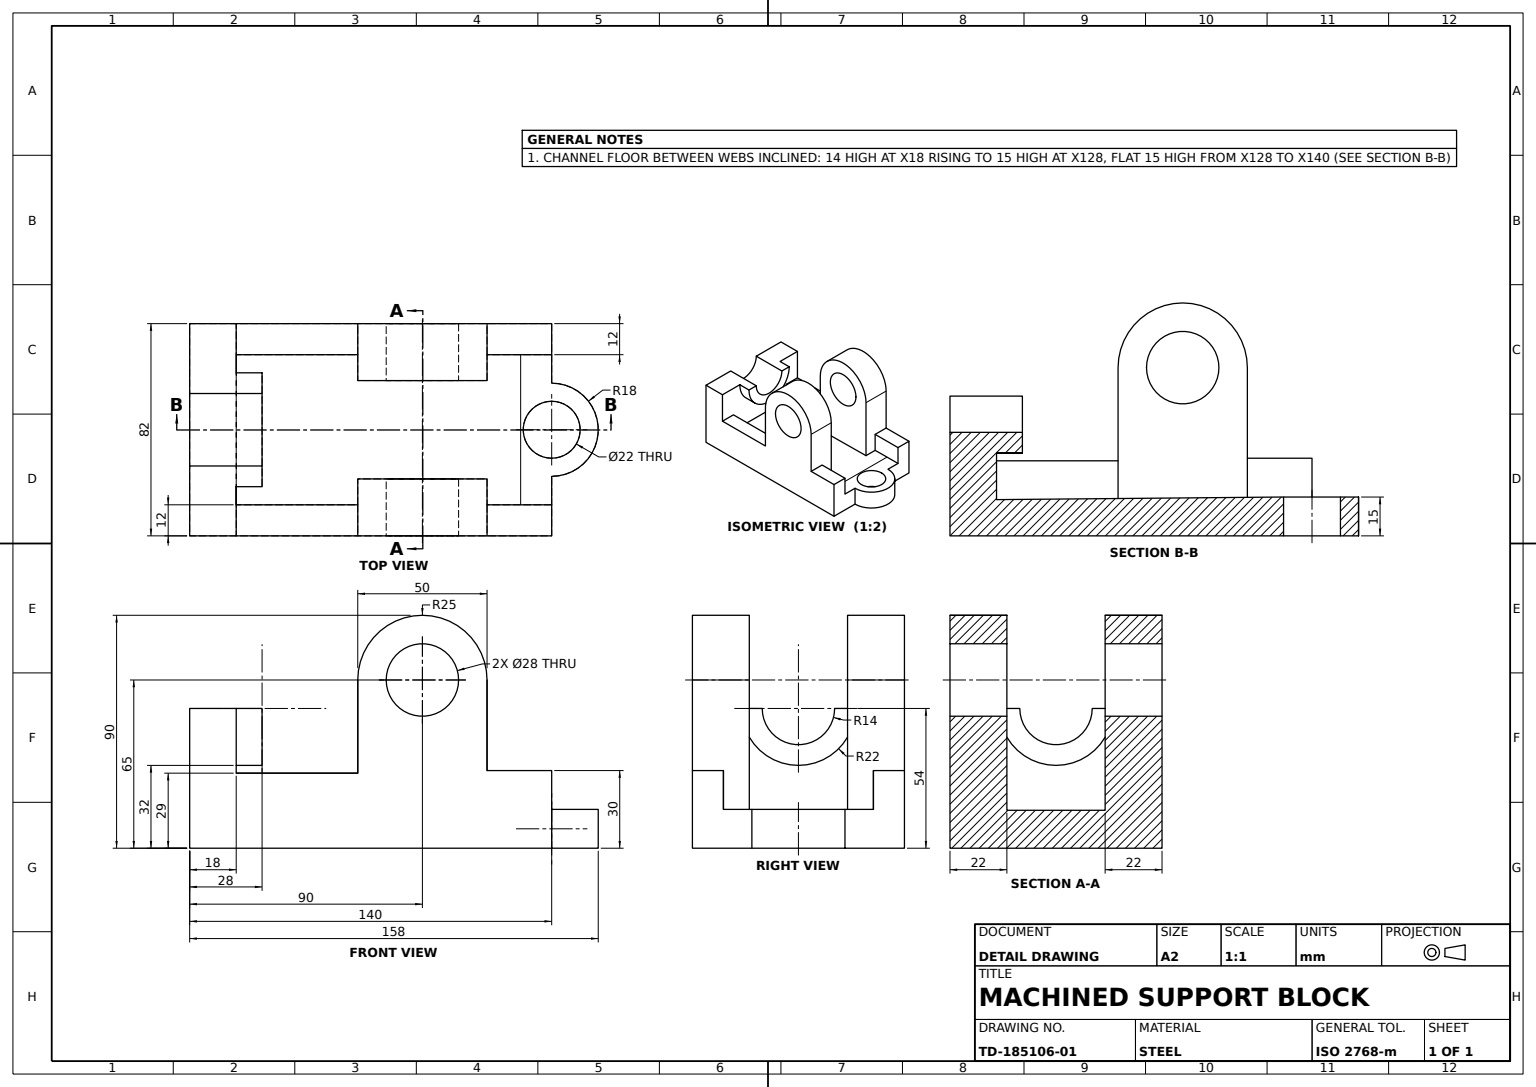
SolidWorks part; units mm, degrees
material "Plain Carbon Steel"
ref_plane "Front Plane" through (0, 0, 0) normal (0, 0, 1) x (1, 0, 0)
ref_plane "Top Plane" through (0, 0, 0) normal (0, 1, 0) x (1, 0, 0)
ref_plane "Right Plane" through (0, 0, 0) normal (1, 0, 0) x (0, 0, -1)
sketch "Base Profile Sketch" plane through (0, 0, 0) normal (0, 0, 1) x (1, 0, 0)
  line L0 (0, 0) -> (140, 0)
  line L1 (140, 0) -> (140, 30)
  line L2 (140, 30) -> (128, 30)
  line L3 (128, 30) -> (128, 15)
  line L5 (0, 15) -> (0, 0)
  line L6 (0, 0) -> (0, 54)
  line L7 (0, 54) -> (18, 54)
  line L8 (18, 54) -> (18, 14)
  line L9 (18, 14) -> (128, 15)
  dimension "D1" = 140
  dimension "D2" = 18
  dimension "D3" = 128
  dimension "D4" = 14
  dimension "D5" = 15
  dimension "D6" = 54
extrude "Base Block" add sketch "Base Profile Sketch" along normal blind 82 contours L9 L8 L7 L6 L5 L0 L1 L2 L3
sketch "Pocket 1 Sketch" plane through (128, 0, 0) normal (-1, 0, 0) x (0, 0, 1)
  line L0 (0, 30) -> (0, 15)
  line L1 (0, 0) -> (0, 54) construction
  line L2 (0, 15) -> (82, 15)
  line L3 (82, 0) -> (82, 54) construction
  line L4 (82, 15) -> (82, 30)
  line L5 (82, 30) -> (0, 30)
  dimension "D1" = 15
extrude "Pocket Cut 1" cut sketch "Pocket 1 Sketch" against normal blind 82
sketch "Pocket 2 Sketch" plane through (0, 15, 0) normal (0, 1, 0) x (1, 0, 0)
  line L0 (128, 0) -> (140, 0)
  line L1 (140, 0) -> (140, -82)
  line L2 (140, -82) -> (128, -82)
  line L3 (128, -82) -> (128, 0)
extrude "Pocket Cut 2" cut sketch "Pocket 2 Sketch" against normal blind 82
sketch "Pad Sketch" plane through (0, 0, 82) normal (0, 0, 1) x (1, 0, 0)
  line L0 (128, 0) -> (140, 0)
  line L1 (140, 0) -> (140, 15)
  line L2 (140, 15) -> (128, 15)
  line L3 (128, 0) -> (128, 15) construction
  line L4 (18, 14) -> (128, 15) construction
  line L5 (128, 15) -> (128, 0)
  line L6 (18, 54) -> (18, 14) construction
  dimension "D1" = 122
extrude "Full Width Pad" add sketch "Pad Sketch" against normal blind 82
sketch "Lug 1 Sketch" plane through (0, 0, 82) normal (0, 0, 1) x (1, 0, 0)
  line L0 (0, 0) -> (90, 0)
  line L1 (0, 0) -> (140, 0) construction
  line L2 (90, 14.6545) -> (90, 15)
  line L3 (140, 0) -> (140, 15) construction
  line L4 (65, 65) -> (65, 14.4273)
  line L5 (18, 14) -> (128, 15) construction
  line L6 (115, 65) -> (115, 14.8818)
  line L7 (115, 14.8818) -> (65, 14.4273)
  arc A0 (115, 65) -> (65, 65) centre (90, 65) ccw
  dimension "D1" = 25
  dimension "D2" = 50
  dimension "D3" = 15
  dimension "D4" = 65
extrude "Lug 1" add sketch "Lug 1 Sketch" against normal blind 22
sketch "Lug 2 Sketch" plane through (0, 0, 0) normal (0, 0, -1) x (-1, 0, 0)
  line L3 (-115, 65) -> (-115, 14.8818)
  line L4 (-18, 14) -> (-128, 15) construction
  line L5 (-115, 65) -> (-115, 14.8818) construction
  line L6 (-115, 14.8818) -> (-65, 14.4273)
  line L7 (-65, 14.4273) -> (-65, 65)
  arc A0 (-65, 65) -> (-115, 65) centre (-90, 65) ccw
extrude "Lug 2" add sketch "Lug 2 Sketch" against normal blind 22
sketch "Web 1 Sketch" plane through (0, 0, 0) normal (0, 0, -1) x (-1, 0, 0)
  line L0 (-18, 14) -> (-18, 29)
  line L1 (-18, 54) -> (-18, 14) construction
  line L2 (-18, 29) -> (-65, 29)
  line L3 (-65, 14.4273) -> (-65, 65) construction
  line L4 (-65, 29) -> (-65, 14.4273)
  line L5 (-65, 14.4273) -> (-18, 14)
  line L6 (-140, 15) -> (-128, 15) construction
  dimension "D1" = 14
extrude "Web 1" add sketch "Web 1 Sketch" against normal blind 12
sketch "Web 2 Sketch" plane through (0, 0, 0) normal (0, 0, -1) x (-1, 0, 0)
  line L0 (-140, 15) -> (-140, 30)
  line L1 (-140, 30) -> (-115, 30)
  line L2 (-115, 65) -> (-115, 14.8818) construction
  line L3 (-115, 30) -> (-115, 14.8818)
  line L4 (-115, 14.8818) -> (-140, 15)
  line L6 (-18, 29) -> (-65, 29) construction
  dimension "D1" = 1
extrude "Web 2" add sketch "Web 2 Sketch" against normal blind 12
sketch "Web 3 Sketch" plane through (0, 0, 82) normal (0, 0, 1) x (1, 0, 0)
  line L0 (115, 30) -> (115, 14.8818)
  line L1 (115, 14.8818) -> (140, 15)
  line L2 (140, 15) -> (140, 30)
  line L3 (140, 30) -> (115, 30)
extrude "Web 3" add sketch "Web 3 Sketch" against normal blind 12
sketch "Web 4 Sketch" plane through (0, 0, 82) normal (0, 0, 1) x (1, 0, 0)
  line L0 (18, 14) -> (18, 29)
  line L1 (18, 29) -> (65, 29)
  line L2 (65, 29) -> (65, 14.4273)
  line L3 (65, 14.4273) -> (18, 14)
extrude "Web 4" add sketch "Web 4 Sketch" against normal blind 12
sketch "Lug Bore Sketch" plane through (0, 0, 82) normal (0, 0, 1) x (1, 0, 0)
  circle A0 centre (90, 65) radius 14
  dimension "D1" = 28
extrude "Lug Bore" cut sketch "Lug Bore Sketch" against normal blind 100
sketch "Ear Boss Sketch" plane through (0, 15, 0) normal (0, 1, 0) x (1, 0, 0)
  line L0 (140, -12) -> (140, -70) construction
  line L1 (140, -23) -> (140, -59)
  arc A0 (140, -59) -> (140, -23) centre (140, -41) ccw
  dimension "D1" = 18
extrude "Ear Boss" add sketch "Ear Boss Sketch" against normal blind 15
sketch "Ear Hole Sketch" plane through (0, 15, 0) normal (0, 1, 0) x (1, 0, 0)
  circle A0 centre (140, -41) radius 11
  dimension "D1" = 22
extrude "Ear Hole" cut sketch "Ear Hole Sketch" against normal blind 15
sketch "Side Boss Sketch" plane through (18, 0, 0) normal (1, 0, 0) x (0, 0, -1)
  line L0 (-82, 54) -> (0, 54) construction
  line L1 (-63, 54) -> (-19, 54)
  arc A0 (-63, 54) -> (-19, 54) centre (-41, 54) ccw
  dimension "D1" = 22
extrude "Side Boss" add sketch "Side Boss Sketch" along normal blind 10
sketch "Bearing Seat Sketch" plane through (0, 0, 0) normal (-1, 0, 0) x (0, 0, 1)
  line L0 (82, 54) -> (0, 54) construction
  line L1 (27, 54) -> (55, 54)
  arc A0 (27, 54) -> (55, 54) centre (41, 54) ccw
  dimension "D1" = 14
extrude "Bearing Seat Cut" cut sketch "Bearing Seat Sketch" against normal blind 28
